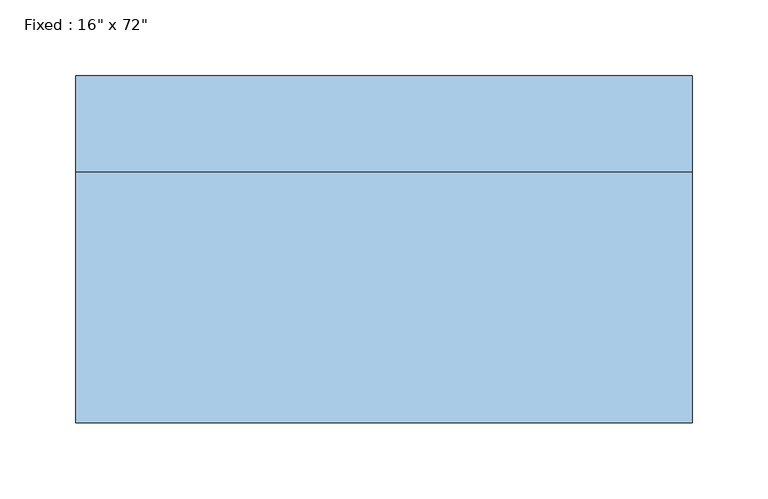
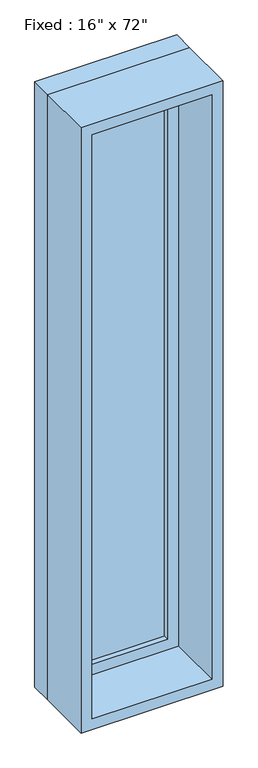
"""IFC4 building model written with IfcOpenShell, lengths in millimetres: window geometry."""

from ifc_helpers import new_model, si_unit, frame, origin, place, context, project, spatial, polyline, outline, extrude, source, transform, mapped, element, save


def window_373d1f99(model_context):
    return source(origin(), model_context, "Body", "SweptSolid", [
        extrude(outline(polyline([(101.6, 66.675), (-177.8, 66.675), (-177.8, 79.375), (101.6, 79.375), (101.6, 66.675)])), frame((0.0, 0.0, 368.3), z_axis=(0.0, 0.0, 1.0), x_axis=(1.0, 0.0, 0.0)), (0.0, 0.0, 1.0), 1701.8),
        extrude(outline(polyline([(2114.55, -222.25), (323.85, -222.25), (323.85, 146.05), (2114.55, 146.05), (2114.55, -222.25)]), holes=[polyline([(2070.1, -177.8), (2070.1, 101.6), (368.3, 101.6), (368.3, -177.8), (2070.1, -177.8)])]), frame((0.0, 50.8, 0.0), z_axis=(0.0, 1.0, 0.0), x_axis=(0.0, 0.0, 1.0)), (0.0, 0.0, 1.0), 44.45),
        extrude(outline(polyline([(2133.6, -241.3), (304.8, -241.3), (304.8, 165.1), (2133.6, 165.1), (2133.6, -241.3)]), holes=[polyline([(2101.85, -209.55), (2101.85, 133.35), (336.55, 133.35), (336.55, -209.55), (2101.85, -209.55)])]), frame((0.0, -114.3, 0.0), z_axis=(0.0, 1.0, 0.0), x_axis=(0.0, 0.0, 1.0)), (0.0, 0.0, 1.0), 165.1),
        extrude(outline(polyline([(2133.6, 165.1), (2133.6, -241.3), (304.8, -241.3), (304.8, 165.1), (2133.6, 165.1)]), holes=[polyline([(2114.55, 146.05), (323.85, 146.05), (323.85, -222.25), (2114.55, -222.25), (2114.55, 146.05)])]), frame((0.0, 50.8, 0.0), z_axis=(0.0, 1.0, 0.0), x_axis=(0.0, 0.0, 1.0)), (0.0, 0.0, 1.0), 63.5),
    ])


if __name__ == "__main__":
    model = new_model("IFC4")
    model_context = context("Model", 3, world=origin())
    ifc_project = project(units=[si_unit("LENGTHUNIT", "METRE", prefix="MILLI")], contexts=[model_context])
    site = spatial("IfcSite", under=ifc_project)
    building = spatial("IfcBuilding", under=site)
    placement = place(None, origin())
    window_shape = window_373d1f99(model_context)
    element("IfcWindow", 1, ObjectType="Fixed : 16\" x 72\"", at=placement, inside=building, context=model_context, shape_type="MappedRepresentation", body=[
        mapped(window_shape, transform((0.0, 0.0, 0.0), x_axis=(1.0, 0.0, 0.0), y_axis=(0.0, 1.0, 0.0), z_axis=(0.0, 0.0, 1.0))),
    ])
    save(model, "model.ifc")

# Revit data of these elements
# Type "Fixed : 16\" x 72\""
#   Type Mark = "6"
#   Construction Type Id = "GSP4R"
#   Assembly Code = "B2020100"
#   Analytic Construction = "1/8 in Pilkington single glazing"
#   Visual Light Transmittance = 0.9
#   Solar Heat Gain Coefficient = 0.78
#   Heat Transfer Coefficient (U) = 0.6496 BTU/(h·ft²·°F)
#   Height = 6' - 0"
#   Default Sill Height = 1' - 0"
#   Width = 1' - 4"
#   Window Inset = 0' - 0 3/4"
#   Define Thermal Properties by = 1
#   Define Thermal Properties by = 1
#   Glass Pane Material = Glass
#   Sash Material = Sash
#   Wall Closure = (empty or 0)
# Element 1 (IfcWindow, "Fixed : 16\" x 72\"")
#   Materials on its faces: "Sash", "Glass"
# Materials
#   "Glass": class "Glass", colour RGB 0 128 192, transparency 0.75, Description = "Soda Lime Glass", Cost = 0
#   "Sash": class "Wood", colour RGB 224 178 126, transparency 0, Cost = 0
